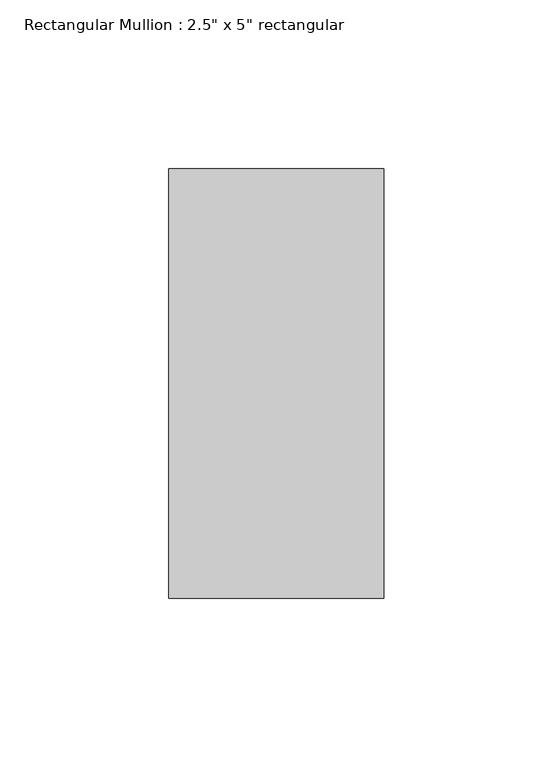
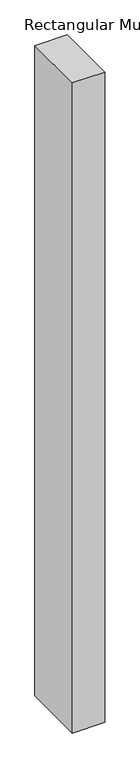
"""IFC4 building model written with IfcOpenShell, lengths in millimetres: member geometry."""

from ifc_helpers import new_model, si_unit, frame, origin, place, context, project, spatial, polyline, outline, extrude, source, transform, mapped, element, save


def member_57611c17(model_context):
    return source(origin(), model_context, "Body", "SweptSolid", [
        extrude(outline(polyline([(31.75, 63.5), (31.75, -63.5), (-31.75, -63.5), (-31.75, 63.5), (31.75, 63.5)])), frame((0.0, 0.0, -1341.7662723), z_axis=(0.0, 0.0, 1.0), x_axis=(1.0, 0.0, 0.0)), (0.0, 0.0, 1.0), 1341.7662723),
    ])


if __name__ == "__main__":
    model = new_model("IFC4")
    model_context = context("Model", 3, world=origin())
    ifc_project = project(units=[si_unit("LENGTHUNIT", "METRE", prefix="MILLI")], contexts=[model_context])
    site = spatial("IfcSite", under=ifc_project)
    building = spatial("IfcBuilding", under=site)
    placement = place(None, origin())
    member_shape = member_57611c17(model_context)
    element("IfcMember", 1, ObjectType="Rectangular Mullion : 2.5\" x 5\" rectangular", at=placement, inside=building, context=model_context, shape_type="MappedRepresentation", body=[
        mapped(member_shape, transform((0.0, 0.0, 0.0), x_axis=(1.0, 0.0, 0.0), y_axis=(0.0, 1.0, 0.0), z_axis=(0.0, 0.0, 1.0))),
    ])
    save(model, "model.ifc")

# Revit data of these elements
# Type "Rectangular Mullion : 2.5\" x 5\" rectangular"
#   built-in parameter 1007304 = 0.416667 (stored number, unit not read)
#   built-in parameter 1007301 = 0.104167 (stored number, unit not read)
#   built-in parameter 1007300 = 0.104167 (stored number, unit not read)
# Element 1 (IfcMember, "Rectangular Mullion : 2.5\" x 5\" rectangular")
#   Materials on its faces: "Aluminum"
# Materials
#   "Aluminum": class "Metal", colour RGB 247 247 247, transparency 0, Description = "Aluminum 6061", Cost = 0
